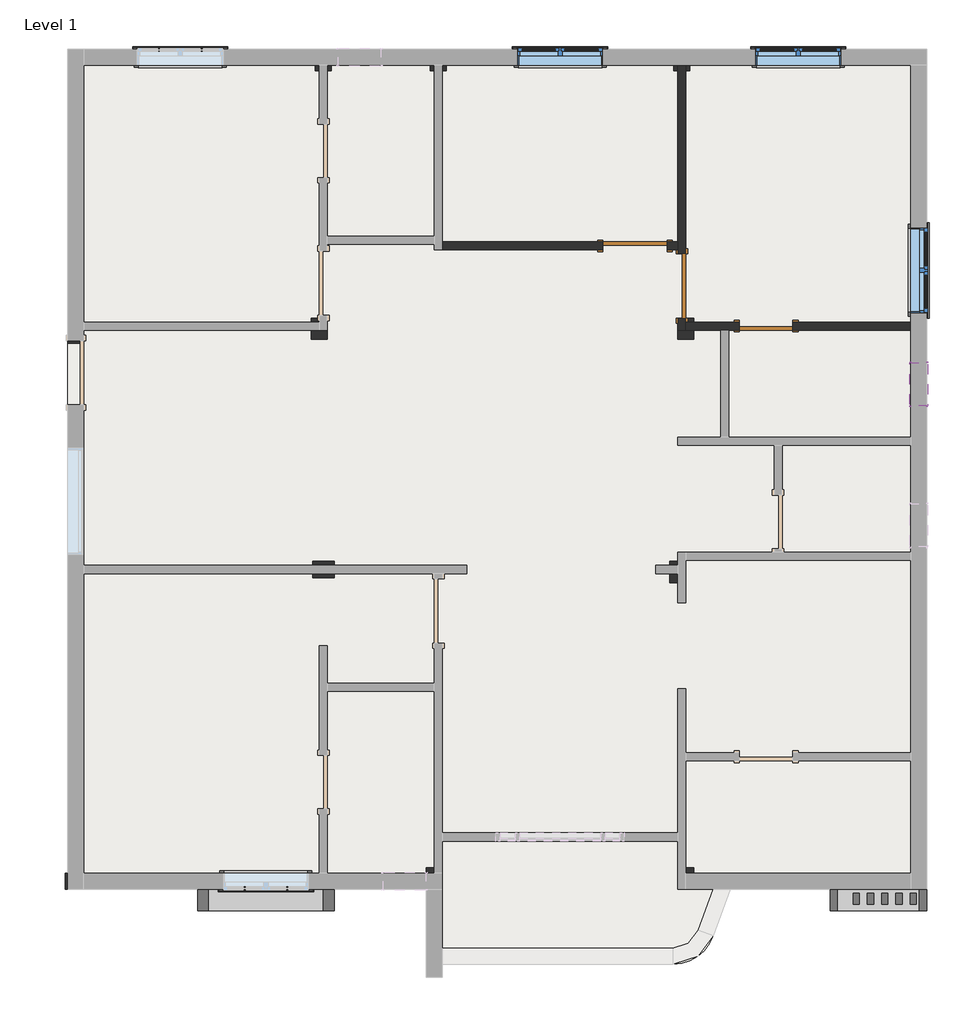
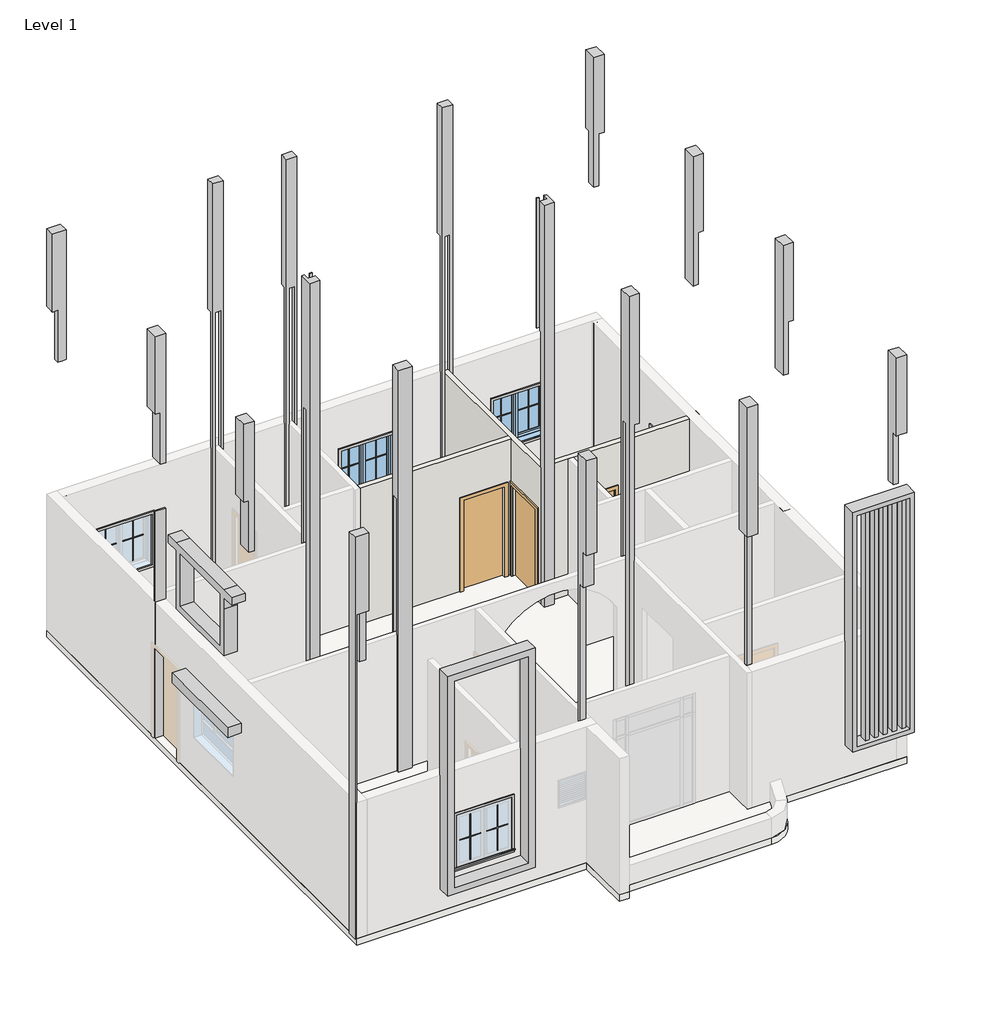
# One storey, part 2 of 2: 21 proxies, 17 columns, 4 windows, 3 doors, 3 walls, 1 slab.
"""IFC4 building model written with IfcOpenShell, lengths in millimetres."""

from ifc_helpers import new_model, si_unit, point, frame, frame_2d, origin, origin_with_axes, place, context, project, spatial, polyline, circle_curve, trimmed, segment, composite_curve, outline, extrude, faceted_brep, transform, mapped, element, save
from components import generic_models_1_generic_models_1_10505d45, muntin_pattern_2x2_muntin_pattern_2x2_4dfeb3f3, muntin_pattern_2x2_muntin_pattern_2x2_e852a7e4, trim_window_exterior_flat_with_sill_7cfdd449, trim_window_interior_flat_picture_frame_f1e0b15b, door_214872d5, door_e5f9f3c4, window_af3140d2, window_f2d8fef0

model = new_model("IFC4")

# Units and contexts
model_context = context("Model", 3, world=origin())
ifc_project = project(units=[si_unit("LENGTHUNIT", "METRE", prefix="MILLI")], contexts=[model_context])

# Site, building, storey
site = spatial("IfcSite", under=ifc_project)
building = spatial("IfcBuilding", under=site)
storey = spatial("IfcBuildingStorey", under=building, Name="Level 1", Elevation=0.0)

# Proxies
placement = place(None, origin())
generic_models_1_generic_models_1_shape = generic_models_1_generic_models_1_10505d45(model_context)
element("IfcBuildingElementProxy", 1, Name="Generic Models 1 : Generic Models 1", ObjectType="Generic Models 1 : Generic Models 1", at=placement, inside=storey, context=model_context, shape_type="MappedRepresentation", body=[
    mapped(generic_models_1_generic_models_1_shape, transform((0.0, 0.0, 0.0), x_axis=(1.0, 0.0, 0.0), y_axis=(0.0, 1.0, 0.0), z_axis=(0.0, 0.0, 1.0))),
])
muntin_pattern_2x2_muntin_pattern_2x2_shape = muntin_pattern_2x2_muntin_pattern_2x2_4dfeb3f3(model_context)
element("IfcBuildingElementProxy", 2, Name="Muntin Pattern_2x2 : Muntin Pattern_2x2", ObjectType="Muntin Pattern_2x2 : Muntin Pattern_2x2", at=placement, inside=storey, context=model_context, shape_type="MappedRepresentation", body=[
    mapped(muntin_pattern_2x2_muntin_pattern_2x2_shape, transform((-13598.9803125, 13522.091018, 984.25), x_axis=(1.0, 0.0, 0.0), y_axis=(0.0, 1.0, 0.0), z_axis=(0.0, 0.0, 1.0))),
])
element("IfcBuildingElementProxy", 3, Name="Muntin Pattern_2x2 : Muntin Pattern_2x2", ObjectType="Muntin Pattern_2x2 : Muntin Pattern_2x2", at=placement, inside=storey, context=model_context, shape_type="MappedRepresentation", body=[
    mapped(muntin_pattern_2x2_muntin_pattern_2x2_shape, transform((-8188.7803125, 13522.091018, 984.25), x_axis=(1.0, 0.0, 0.0), y_axis=(0.0, 1.0, 0.0), z_axis=(0.0, 0.0, 1.0))),
])
element("IfcBuildingElementProxy", 4, Name="Muntin Pattern_2x2 : Muntin Pattern_2x2", ObjectType="Muntin Pattern_2x2 : Muntin Pattern_2x2", at=placement, inside=storey, context=model_context, shape_type="MappedRepresentation", body=[
    mapped(muntin_pattern_2x2_muntin_pattern_2x2_shape, transform((-4797.8803125, 13522.091018, 984.25), x_axis=(1.0, 0.0, 0.0), y_axis=(0.0, 1.0, 0.0), z_axis=(0.0, 0.0, 1.0))),
])
element("IfcBuildingElementProxy", 5, Name="Muntin Pattern_2x2 : Muntin Pattern_2x2", ObjectType="Muntin Pattern_2x2 : Muntin Pattern_2x2", at=placement, inside=storey, context=model_context, shape_type="MappedRepresentation", body=[
    mapped(muntin_pattern_2x2_muntin_pattern_2x2_shape, transform((-2675.3928125, 10685.228518, 984.25), x_axis=(0.0, -1.0, 0.0), y_axis=(1.0, 0.0, 0.0), z_axis=(0.0, 0.0, 1.0))),
])
element("IfcBuildingElementProxy", 6, Name="Muntin Pattern_2x2 : Muntin Pattern_2x2", ObjectType="Muntin Pattern_2x2 : Muntin Pattern_2x2", at=placement, inside=storey, context=model_context, shape_type="MappedRepresentation", body=[
    mapped(muntin_pattern_2x2_muntin_pattern_2x2_shape, transform((-11773.3553125, 1577.741018, 984.25), x_axis=(-1.0, 0.0, 0.0), y_axis=(0.0, -1.0, 0.0), z_axis=(0.0, 0.0, 1.0))),
])
muntin_pattern_2x2_muntin_pattern_2x2_2_shape = muntin_pattern_2x2_muntin_pattern_2x2_e852a7e4(model_context)
element("IfcBuildingElementProxy", 7, Name="Muntin Pattern_2x2 : Muntin Pattern_2x2", ObjectType="Muntin Pattern_2x2 : Muntin Pattern_2x2", at=placement, inside=storey, context=model_context, shape_type="MappedRepresentation", body=[
    mapped(muntin_pattern_2x2_muntin_pattern_2x2_2_shape, transform((-12992.5553125, 13522.091018, 984.25), x_axis=(-1.0, 0.0, 0.0), y_axis=(0.0, -1.0, 0.0), z_axis=(0.0, 0.0, 1.0))),
])
element("IfcBuildingElementProxy", 8, Name="Muntin Pattern_2x2 : Muntin Pattern_2x2", ObjectType="Muntin Pattern_2x2 : Muntin Pattern_2x2", at=placement, inside=storey, context=model_context, shape_type="MappedRepresentation", body=[
    mapped(muntin_pattern_2x2_muntin_pattern_2x2_2_shape, transform((-7582.3553125, 13522.091018, 984.25), x_axis=(-1.0, 0.0, 0.0), y_axis=(0.0, -1.0, 0.0), z_axis=(0.0, 0.0, 1.0))),
])
element("IfcBuildingElementProxy", 9, Name="Muntin Pattern_2x2 : Muntin Pattern_2x2", ObjectType="Muntin Pattern_2x2 : Muntin Pattern_2x2", at=placement, inside=storey, context=model_context, shape_type="MappedRepresentation", body=[
    mapped(muntin_pattern_2x2_muntin_pattern_2x2_2_shape, transform((-4191.4553125, 13522.091018, 984.25), x_axis=(-1.0, 0.0, 0.0), y_axis=(0.0, -1.0, 0.0), z_axis=(0.0, 0.0, 1.0))),
])
element("IfcBuildingElementProxy", 10, Name="Muntin Pattern_2x2 : Muntin Pattern_2x2", ObjectType="Muntin Pattern_2x2 : Muntin Pattern_2x2", at=placement, inside=storey, context=model_context, shape_type="MappedRepresentation", body=[
    mapped(muntin_pattern_2x2_muntin_pattern_2x2_2_shape, transform((-2675.3928125, 10078.803518, 984.25), x_axis=(0.0, 1.0, 0.0), y_axis=(-1.0, 0.0, 0.0), z_axis=(0.0, 0.0, 1.0))),
])
element("IfcBuildingElementProxy", 11, Name="Muntin Pattern_2x2 : Muntin Pattern_2x2", ObjectType="Muntin Pattern_2x2 : Muntin Pattern_2x2", at=placement, inside=storey, context=model_context, shape_type="MappedRepresentation", body=[
    mapped(muntin_pattern_2x2_muntin_pattern_2x2_2_shape, transform((-12379.7803125, 1577.741018, 984.25), x_axis=(1.0, 0.0, 0.0), y_axis=(0.0, 1.0, 0.0), z_axis=(0.0, 0.0, 1.0))),
])
trim_window_exterior_flat_with_sill_shape = trim_window_exterior_flat_with_sill_7cfdd449(model_context)
element("IfcBuildingElementProxy", 12, Name="Trim-Window-Exterior-Flat : with Sill", ObjectType="Trim-Window-Exterior-Flat : with Sill", at=placement, inside=storey, context=model_context, shape_type="MappedRepresentation", body=[
    mapped(trim_window_exterior_flat_with_sill_shape, transform((-13295.7678125, 13531.616018, 2133.6), x_axis=(-1.0, 0.0, 0.0), y_axis=(0.0, 0.0, 1.0), z_axis=(0.0, 1.0, 0.0))),
])
element("IfcBuildingElementProxy", 13, Name="Trim-Window-Exterior-Flat : with Sill", ObjectType="Trim-Window-Exterior-Flat : with Sill", at=placement, inside=storey, context=model_context, shape_type="MappedRepresentation", body=[
    mapped(trim_window_exterior_flat_with_sill_shape, transform((-7885.5678125, 13531.616018, 2133.6), x_axis=(-1.0, 0.0, 0.0), y_axis=(0.0, 0.0, 1.0), z_axis=(0.0, 1.0, 0.0))),
])
element("IfcBuildingElementProxy", 14, Name="Trim-Window-Exterior-Flat : with Sill", ObjectType="Trim-Window-Exterior-Flat : with Sill", at=placement, inside=storey, context=model_context, shape_type="MappedRepresentation", body=[
    mapped(trim_window_exterior_flat_with_sill_shape, transform((-4494.6678125, 13531.616018, 2133.6), x_axis=(-1.0, 0.0, 0.0), y_axis=(0.0, 0.0, 1.0), z_axis=(0.0, 1.0, 0.0))),
])
element("IfcBuildingElementProxy", 15, Name="Trim-Window-Exterior-Flat : with Sill", ObjectType="Trim-Window-Exterior-Flat : with Sill", at=placement, inside=storey, context=model_context, shape_type="MappedRepresentation", body=[
    mapped(trim_window_exterior_flat_with_sill_shape, transform((-2665.8678125, 10382.016018, 2133.6), x_axis=(0.0, 1.0, 0.0), y_axis=(0.0, 0.0, 1.0), z_axis=(1.0, 0.0, 0.0))),
])
element("IfcBuildingElementProxy", 16, Name="Trim-Window-Exterior-Flat : with Sill", ObjectType="Trim-Window-Exterior-Flat : with Sill", at=placement, inside=storey, context=model_context, shape_type="MappedRepresentation", body=[
    mapped(trim_window_exterior_flat_with_sill_shape, transform((-12076.5678125, 1568.216018, 2133.6), x_axis=(1.0, 0.0, 0.0), y_axis=(0.0, 0.0, 1.0), z_axis=(0.0, -1.0, 0.0))),
])
trim_window_interior_flat_picture_frame_shape = trim_window_interior_flat_picture_frame_f1e0b15b(model_context)
element("IfcBuildingElementProxy", 17, Name="Trim-Window-Interior-Flat : Picture Frame", ObjectType="Trim-Window-Interior-Flat : Picture Frame", at=placement, inside=storey, context=model_context, shape_type="MappedRepresentation", body=[
    mapped(trim_window_interior_flat_picture_frame_shape, transform((-13295.7678125, 13303.016018, 2133.6), x_axis=(1.0, 0.0, 0.0), y_axis=(0.0, 0.0, 1.0), z_axis=(0.0, -1.0, 0.0))),
])
element("IfcBuildingElementProxy", 18, Name="Trim-Window-Interior-Flat : Picture Frame", ObjectType="Trim-Window-Interior-Flat : Picture Frame", at=placement, inside=storey, context=model_context, shape_type="MappedRepresentation", body=[
    mapped(trim_window_interior_flat_picture_frame_shape, transform((-7885.5678125, 13303.016018, 2133.6), x_axis=(1.0, 0.0, 0.0), y_axis=(0.0, 0.0, 1.0), z_axis=(0.0, -1.0, 0.0))),
])
element("IfcBuildingElementProxy", 19, Name="Trim-Window-Interior-Flat : Picture Frame", ObjectType="Trim-Window-Interior-Flat : Picture Frame", at=placement, inside=storey, context=model_context, shape_type="MappedRepresentation", body=[
    mapped(trim_window_interior_flat_picture_frame_shape, transform((-4494.6678125, 13303.016018, 2133.6), x_axis=(1.0, 0.0, 0.0), y_axis=(0.0, 0.0, 1.0), z_axis=(0.0, -1.0, 0.0))),
])
element("IfcBuildingElementProxy", 20, Name="Trim-Window-Interior-Flat : Picture Frame", ObjectType="Trim-Window-Interior-Flat : Picture Frame", at=placement, inside=storey, context=model_context, shape_type="MappedRepresentation", body=[
    mapped(trim_window_interior_flat_picture_frame_shape, transform((-2894.4678125, 10382.016018, 2133.6), x_axis=(0.0, -1.0, 0.0), y_axis=(0.0, 0.0, 1.0), z_axis=(-1.0, 0.0, 0.0))),
])
element("IfcBuildingElementProxy", 21, Name="Trim-Window-Interior-Flat : Picture Frame", ObjectType="Trim-Window-Interior-Flat : Picture Frame", at=placement, inside=storey, context=model_context, shape_type="MappedRepresentation", body=[
    mapped(trim_window_interior_flat_picture_frame_shape, transform((-12076.5678125, 1796.816018, 2133.6), x_axis=(-1.0, 0.0, 0.0), y_axis=(0.0, 0.0, 1.0), z_axis=(0.0, 1.0, 0.0))),
])

# Columns
element("IfcColumn", 22, ObjectType="Rectangular Column : 9\" x 12\"", at=placement, inside=storey, context=model_context, shape_type="Brep", body=[
    faceted_brep([(-14591.1678125, 13531.616018, 0.0), (-14591.1678125, 13303.016018, 0.0), (-14667.3678125, 13303.016018, 0.0), (-14667.3678125, 13531.616018, 0.0), (-14667.3678125, 13303.016018, 3200.4), (-14667.3678125, 13531.616018, 3200.4), (-14591.1678125, 13303.016018, 3200.4), (-14591.1678125, 13531.616018, 3200.4)], [[[0, 1, 2, 3]], [[3, 2, 4, 5]], [[6, 7, 5, 4]], [[1, 0, 7, 6]], [[2, 1, 6, 4]], [[0, 3, 5, 7]]]),
    faceted_brep([(-14591.1678125, 13531.616018, 9448.8), (-14591.1678125, 13303.016018, 9448.8), (-14591.1678125, 13303.016018, 6400.8), (-14591.1678125, 13417.316018, 6400.8), (-14591.1678125, 13417.316018, 7620.0), (-14591.1678125, 13531.616018, 7620.0), (-14895.9678125, 13303.016018, 9448.8), (-14895.9678125, 13303.016018, 7620.0), (-14781.6678125, 13303.016018, 7620.0), (-14781.6678125, 13303.016018, 6400.8), (-14667.3678125, 13303.016018, 6400.8), (-14895.9678125, 13531.616018, 9448.8), (-14895.9678125, 13531.616018, 7620.0), (-14895.9678125, 13417.316018, 7620.0), (-14781.6678125, 13417.316018, 6400.8), (-14667.3678125, 13417.316018, 6400.8), (-14781.6678125, 13417.316018, 7620.0)], [[[0, 1, 2, 3, 4, 5]], [[1, 6, 7, 8, 9, 10, 2]], [[6, 11, 12, 13, 7]], [[11, 0, 5, 12]], [[1, 0, 11, 6]], [[10, 9, 14, 15]], [[2, 10, 15, 3]], [[8, 16, 14, 9]], [[16, 8, 7, 13]], [[16, 4, 3, 15, 14]], [[4, 16, 13, 12, 5]]]),
])
element("IfcColumn", 23, ObjectType="Rectangular Column : 9\" x 12\"", at=placement, inside=storey, context=model_context, shape_type="Brep", body=[
    faceted_brep([(-11371.7178125, 13226.816018, 0.0), (-11371.7178125, 13303.016018, 0.0), (-11314.5678125, 13303.016018, 0.0), (-11314.5678125, 13226.816018, 0.0), (-11143.1178125, 13226.816018, 9448.8), (-11143.1178125, 13226.816018, 0.0), (-11143.1178125, 13303.016018, 0.0), (-11143.1178125, 13303.016018, 3200.4), (-11143.1178125, 13303.016018, 6400.8), (-11143.1178125, 13417.316018, 6400.8), (-11143.1178125, 13417.316018, 9448.8), (-11257.4178125, 13226.816018, 9448.8), (-11371.7178125, 13226.816018, 9448.8), (-11371.7178125, 13226.816018, 6400.8), (-11314.5678125, 13226.816018, 3200.4), (-11314.5678125, 13226.816018, 6400.8), (-11257.4178125, 13226.816018, 6400.8), (-11200.2678125, 13226.816018, 6400.8), (-11200.2678125, 13226.816018, 3200.4), (-11200.2678125, 13226.816018, 0.0), (-11371.7178125, 13417.316018, 9448.8), (-11371.7178125, 13417.316018, 6400.8), (-11371.7178125, 13303.016018, 6400.8), (-11371.7178125, 13303.016018, 3200.4), (-11314.5678125, 13303.016018, 3200.4), (-11200.2678125, 13303.016018, 0.0), (-11200.2678125, 13303.016018, 3200.4), (-11314.5678125, 13303.016018, 6400.8), (-11200.2678125, 13303.016018, 6400.8)], [[[0, 1, 2, 3]], [[4, 5, 6, 7, 8, 9, 10]], [[5, 4, 11, 12, 13, 0, 3, 14, 15, 16, 17, 18, 19]], [[0, 13, 12, 20, 21, 22, 23, 1]], [[12, 11, 4, 10, 20]], [[1, 23, 24, 2]], [[3, 2, 24, 14]], [[25, 19, 18, 26]], [[6, 5, 19, 25]], [[7, 6, 25, 26]], [[23, 22, 27, 24]], [[27, 22, 21, 9, 8, 28]], [[27, 15, 14, 24]], [[17, 28, 26, 18]], [[15, 27, 28, 17, 16]], [[8, 7, 26, 28]], [[10, 9, 21, 20]]]),
])
element("IfcColumn", 24, ObjectType="Rectangular Column : 9\" x 12\"", at=placement, inside=storey, context=model_context, shape_type="Brep", body=[
    faceted_brep([(-9733.4178125, 13226.816018, 0.0), (-9733.4178125, 13303.016018, 0.0), (-9676.2678125, 13303.016018, 0.0), (-9676.2678125, 13226.816018, 0.0), (-9504.8178125, 13226.816018, 9448.8), (-9504.8178125, 13226.816018, 0.0), (-9504.8178125, 13303.016018, 0.0), (-9504.8178125, 13303.016018, 3200.4), (-9504.8178125, 13303.016018, 6400.8), (-9504.8178125, 13417.316018, 6400.8), (-9504.8178125, 13417.316018, 9448.8), (-9733.4178125, 13226.816018, 9448.8), (-9676.2678125, 13226.816018, 3200.4), (-9676.2678125, 13226.816018, 6400.8), (-9561.9678125, 13226.816018, 6400.8), (-9561.9678125, 13226.816018, 3200.4), (-9561.9678125, 13226.816018, 0.0), (-9733.4178125, 13417.316018, 9448.8), (-9733.4178125, 13417.316018, 6400.8), (-9733.4178125, 13303.016018, 6400.8), (-9733.4178125, 13303.016018, 3200.4), (-9676.2678125, 13303.016018, 3200.4), (-9561.9678125, 13303.016018, 0.0), (-9561.9678125, 13303.016018, 3200.4), (-9676.2678125, 13303.016018, 6400.8), (-9561.9678125, 13303.016018, 6400.8)], [[[0, 1, 2, 3]], [[4, 5, 6, 7, 8, 9, 10]], [[5, 4, 11, 0, 3, 12, 13, 14, 15, 16]], [[0, 11, 17, 18, 19, 20, 1]], [[11, 4, 10, 17]], [[1, 20, 21, 2]], [[3, 2, 21, 12]], [[22, 16, 15, 23]], [[6, 5, 16, 22]], [[7, 6, 22, 23]], [[20, 19, 24, 21]], [[24, 19, 18, 9, 8, 25]], [[24, 13, 12, 21]], [[14, 25, 23, 15]], [[13, 24, 25, 14]], [[8, 7, 23, 25]], [[10, 9, 18, 17]]]),
])
element("IfcColumn", 25, ObjectType="Rectangular Column : 9\" x 12\"", at=placement, inside=storey, context=model_context, shape_type="Brep", body=[
    faceted_brep([(-6266.3178125, 13226.816018, 0.0), (-6266.3178125, 13303.016018, 0.0), (-6209.1678125, 13303.016018, 0.0), (-6209.1678125, 13226.816018, 0.0), (-6037.7178125, 13226.816018, 9448.8), (-6037.7178125, 13226.816018, 6400.8), (-6037.7178125, 13226.816018, 0.0), (-6037.7178125, 13303.016018, 0.0), (-6037.7178125, 13303.016018, 3200.4), (-6037.7178125, 13303.016018, 6400.8), (-6037.7178125, 13417.316018, 6400.8), (-6037.7178125, 13417.316018, 9448.8), (-6152.0178125, 13226.816018, 9448.8), (-6266.3178125, 13226.816018, 9448.8), (-6209.1678125, 13226.816018, 3200.4), (-6209.1678125, 13226.816018, 6400.8), (-6152.0178125, 13226.816018, 6400.8), (-6094.8678125, 13226.816018, 6400.8), (-6094.8678125, 13226.816018, 3200.4), (-6094.8678125, 13226.816018, 0.0), (-6266.3178125, 13417.316018, 9448.8), (-6266.3178125, 13417.316018, 6400.8), (-6266.3178125, 13303.016018, 6400.8), (-6266.3178125, 13303.016018, 3200.4), (-6209.1678125, 13303.016018, 3200.4), (-6094.8678125, 13303.016018, 0.0), (-6094.8678125, 13303.016018, 3200.4), (-6209.1678125, 13303.016018, 6400.8), (-6094.8678125, 13303.016018, 6400.8)], [[[0, 1, 2, 3]], [[4, 5, 6, 7, 8, 9, 10, 11]], [[6, 5, 4, 12, 13, 0, 3, 14, 15, 16, 17, 18, 19]], [[0, 13, 20, 21, 22, 23, 1]], [[13, 12, 4, 11, 20]], [[1, 23, 24, 2]], [[3, 2, 24, 14]], [[25, 19, 18, 26]], [[7, 6, 19, 25]], [[8, 7, 25, 26]], [[23, 22, 27, 24]], [[27, 22, 21, 10, 9, 28]], [[27, 15, 14, 24]], [[17, 28, 26, 18]], [[15, 27, 28, 17, 16]], [[9, 8, 26, 28]], [[11, 10, 21, 20]]]),
])
element("IfcColumn", 26, ObjectType="Rectangular Column : 9\" x 12\"", at=placement, inside=storey, context=model_context, shape_type="Brep", body=[
    faceted_brep([(-2665.8678125, 13226.816018, 0.0), (-2894.4678125, 13226.816018, 0.0), (-2894.4678125, 13303.016018, 0.0), (-2665.8678125, 13303.016018, 0.0), (-2894.4678125, 13303.016018, 3200.4), (-2665.8678125, 13303.016018, 3200.4), (-2665.8678125, 13226.816018, 3200.4), (-2894.4678125, 13226.816018, 3200.4)], [[[0, 1, 2, 3]], [[3, 2, 4, 5]], [[6, 5, 4, 7]], [[0, 3, 5, 6]], [[1, 0, 6, 7]], [[2, 1, 7, 4]]]),
    faceted_brep([(-2894.4678125, 13531.616018, 9448.8), (-2665.8678125, 13531.616018, 9448.8), (-2665.8678125, 13531.616018, 7620.0), (-2894.4678125, 13531.616018, 7620.0), (-2665.8678125, 13226.816018, 9448.8), (-2665.8678125, 13226.816018, 7620.0), (-2665.8678125, 13417.316018, 7620.0), (-2894.4678125, 13226.816018, 9448.8), (-2894.4678125, 13226.816018, 6400.8), (-2780.1678125, 13226.816018, 6400.8), (-2780.1678125, 13226.816018, 7620.0), (-2894.4678125, 13417.316018, 7620.0), (-2894.4678125, 13417.316018, 6400.8), (-2894.4678125, 13303.016018, 6400.8), (-2780.1678125, 13417.316018, 6400.8), (-2780.1678125, 13303.016018, 6400.8), (-2780.1678125, 13417.316018, 7620.0)], [[[0, 1, 2, 3]], [[1, 4, 5, 6, 2]], [[4, 7, 8, 9, 10, 5]], [[7, 0, 3, 11, 12, 13, 8]], [[1, 0, 7, 4]], [[13, 12, 14, 15]], [[8, 13, 15, 9]], [[12, 11, 16, 14]], [[3, 2, 6, 16, 11]], [[16, 10, 9, 15, 14]], [[10, 16, 6, 5]]]),
])
element("IfcColumn", 27, ObjectType="Rectangular Column : 9\" x 12\"", at=placement, inside=storey, context=model_context, shape_type="Brep", body=[
    faceted_brep([(-14895.9678125, 9645.416018, 0.0), (-14667.3678125, 9645.416018, 0.0), (-14667.3678125, 9531.116018, 0.0), (-14667.3678125, 9340.616018, 0.0), (-14895.9678125, 9340.616018, 0.0), (-14895.9678125, 9378.716018, 3200.4), (-14667.3678125, 9378.716018, 3200.4), (-14667.3678125, 9531.116018, 3200.4), (-14667.3678125, 9645.416018, 3200.4), (-14895.9678125, 9645.416018, 3200.4), (-14895.9678125, 9378.716018, 5334.0), (-14667.3678125, 9378.716018, 5334.0), (-14895.9678125, 9340.616018, 5334.0), (-14667.3678125, 9340.616018, 5334.0)], [[[0, 1, 2, 3, 4]], [[5, 6, 7, 8, 9]], [[6, 5, 10, 11]], [[11, 10, 12, 13]], [[1, 0, 9, 8]], [[3, 2, 1, 8, 7, 6, 11, 13]], [[4, 3, 13, 12]], [[0, 4, 12, 10, 5, 9]]]),
    faceted_brep([(-14895.9678125, 9645.416018, 9448.8), (-14667.3678125, 9645.416018, 9448.8), (-14667.3678125, 9645.416018, 6400.8), (-14781.6678125, 9645.416018, 6400.8), (-14781.6678125, 9645.416018, 7620.0), (-14895.9678125, 9645.416018, 7620.0), (-14667.3678125, 9340.616018, 9448.8), (-14667.3678125, 9340.616018, 6400.8), (-14895.9678125, 9340.616018, 9448.8), (-14895.9678125, 9340.616018, 7620.0), (-14781.6678125, 9340.616018, 7620.0), (-14781.6678125, 9340.616018, 6400.8)], [[[0, 1, 2, 3, 4, 5]], [[1, 6, 7, 2]], [[6, 8, 9, 10, 11, 7]], [[8, 0, 5, 9]], [[1, 0, 8, 6]], [[2, 7, 11, 3]], [[10, 4, 3, 11]], [[4, 10, 9, 5]]]),
])
element("IfcColumn", 28, ObjectType="Rectangular Column : 9\" x 12\"", at=placement, inside=storey, context=model_context, shape_type="Brep", body=[
    faceted_brep([(-11200.2678125, 9397.766018, 0.0), (-11428.8678125, 9397.766018, 0.0), (-11428.8678125, 9531.116018, 0.0), (-11314.5678125, 9531.116018, 0.0), (-11200.2678125, 9531.116018, 0.0), (-11200.2678125, 9397.766018, 9448.8), (-11200.2678125, 9531.116018, 3200.4), (-11200.2678125, 9531.116018, 6400.8), (-11200.2678125, 9569.216018, 6400.8), (-11200.2678125, 9569.216018, 9448.8), (-11428.8678125, 9397.766018, 9448.8), (-11428.8678125, 9702.566018, 9448.8), (-11428.8678125, 9702.566018, 0.0), (-11428.8678125, 9645.416018, 0.0), (-11428.8678125, 9645.416018, 3200.4), (-11428.8678125, 9645.416018, 6400.8), (-11428.8678125, 9531.116018, 6400.8), (-11428.8678125, 9531.116018, 3200.4), (-11314.5678125, 9702.566018, 0.0), (-11314.5678125, 9702.566018, 3200.4), (-11314.5678125, 9645.416018, 3200.4), (-11314.5678125, 9645.416018, 0.0), (-11314.5678125, 9531.116018, 3200.4), (-11314.5678125, 9702.566018, 6400.8), (-11314.5678125, 9645.416018, 6400.8), (-11314.5678125, 9531.116018, 6400.8), (-11314.5678125, 9569.216018, 6400.8), (-11257.4178125, 9569.216018, 6400.8), (-11371.7178125, 9645.416018, 6400.8), (-11371.7178125, 9569.216018, 6400.8), (-11371.7178125, 9702.566018, 6400.8), (-11371.7178125, 9702.566018, 9448.8), (-11371.7178125, 9569.216018, 9448.8), (-11257.4178125, 9569.216018, 9448.8)], [[[0, 1, 2, 3, 4]], [[5, 0, 4, 6, 7, 8, 9]], [[1, 0, 5, 10]], [[11, 12, 13, 14, 15, 16, 17, 2, 1, 10]], [[18, 19, 20, 21]], [[4, 3, 22, 6]], [[3, 2, 17, 22]], [[13, 21, 20, 14]], [[12, 18, 21, 13]], [[19, 23, 24, 20]], [[7, 25, 26, 27, 8]], [[25, 7, 6, 22]], [[16, 25, 22, 17]], [[15, 14, 20, 24, 28]], [[25, 16, 15, 28, 29, 26]], [[28, 30, 31, 32, 29]], [[30, 28, 24, 23]], [[29, 32, 33, 27, 26]], [[9, 8, 27, 33]], [[12, 11, 31, 30, 23, 19, 18]], [[10, 5, 9, 33, 32, 31, 11]]]),
    faceted_brep([(-11200.2678125, 9702.566018, 9448.8), (-11200.2678125, 9702.566018, 6400.8), (-11257.4178125, 9702.566018, 6400.8), (-11257.4178125, 9702.566018, 9448.8), (-11257.4178125, 9683.516018, 9448.8), (-11200.2678125, 9683.516018, 9448.8), (-11257.4178125, 9683.516018, 6400.8), (-11200.2678125, 9683.516018, 6400.8)], [[[0, 1, 2, 3]], [[0, 3, 4, 5]], [[3, 2, 6, 4]], [[7, 5, 4, 6]], [[2, 1, 7, 6]], [[1, 0, 5, 7]]]),
])
element("IfcColumn", 29, ObjectType="Rectangular Column : 9\" x 12\"", at=placement, inside=storey, context=model_context, shape_type="Brep", body=[
    faceted_brep([(-5980.5678125, 9397.766018, 0.0), (-6209.1678125, 9397.766018, 0.0), (-6209.1678125, 9531.116018, 0.0), (-6094.8678125, 9531.116018, 0.0), (-5980.5678125, 9531.116018, 0.0), (-5980.5678125, 9702.566018, 9448.8), (-5980.5678125, 9702.566018, 0.0), (-6094.8678125, 9702.566018, 0.0), (-6094.8678125, 9702.566018, 2133.6), (-6094.8678125, 9702.566018, 3200.4), (-6094.8678125, 9702.566018, 5334.0), (-6094.8678125, 9702.566018, 6400.8), (-6037.7178125, 9702.566018, 6400.8), (-6037.7178125, 9702.566018, 9448.8), (-5980.5678125, 9397.766018, 9448.8), (-5980.5678125, 9531.116018, 3200.4), (-5980.5678125, 9531.116018, 6400.8), (-5980.5678125, 9645.416018, 6400.8), (-5980.5678125, 9645.416018, 3200.4), (-5980.5678125, 9645.416018, 0.0), (-6209.1678125, 9397.766018, 9448.8), (-6209.1678125, 9569.216018, 9448.8), (-6209.1678125, 9569.216018, 6400.8), (-6209.1678125, 9531.116018, 6400.8), (-6209.1678125, 9531.116018, 3200.4), (-6094.8678125, 9645.416018, 0.0), (-6094.8678125, 9645.416018, 3200.4), (-6094.8678125, 9531.116018, 3200.4), (-6094.8678125, 9645.416018, 6400.8), (-6094.8678125, 9683.516018, 6400.8), (-6094.8678125, 9531.116018, 6400.8), (-6094.8678125, 9569.216018, 6400.8), (-6037.7178125, 9645.416018, 6400.8), (-6037.7178125, 9569.216018, 6400.8), (-6037.7178125, 9569.216018, 9448.8), (-6037.7178125, 9683.516018, 6400.8), (-6037.7178125, 9683.516018, 9448.8)], [[[0, 1, 2, 3, 4]], [[5, 6, 7, 8, 9, 10, 11, 12, 13]], [[6, 5, 14, 0, 4, 15, 16, 17, 18, 19]], [[1, 0, 14, 20]], [[1, 20, 21, 22, 23, 24, 2]], [[8, 7, 25, 26, 9]], [[3, 2, 24, 27]], [[4, 3, 27, 15]], [[25, 19, 18, 26]], [[7, 6, 19, 25]], [[10, 9, 26, 28, 29, 11]], [[30, 23, 22, 31]], [[23, 30, 27, 24]], [[30, 16, 15, 27]], [[18, 17, 32, 28, 26]], [[16, 30, 31, 33, 32, 17]], [[22, 21, 34, 33, 31]], [[29, 28, 32, 35]], [[33, 34, 36, 35, 32]], [[12, 35, 36, 13]], [[35, 12, 11, 29]], [[14, 5, 13, 36, 34, 21, 20]]]),
    faceted_brep([(-6209.1678125, 9702.566018, 9448.8), (-6209.1678125, 9683.516018, 9448.8), (-6152.0178125, 9683.516018, 9448.8), (-6152.0178125, 9702.566018, 9448.8), (-6209.1678125, 9683.516018, 6400.8), (-6152.0178125, 9683.516018, 6400.8), (-6209.1678125, 9702.566018, 6400.8), (-6152.0178125, 9702.566018, 6400.8)], [[[0, 1, 2, 3]], [[1, 4, 5, 2]], [[4, 6, 7, 5]], [[7, 3, 2, 5]], [[0, 6, 4, 1]], [[6, 0, 3, 7]]]),
])
element("IfcColumn", 30, ObjectType="Rectangular Column : 9\" x 12\"", at=placement, inside=storey, context=model_context, shape_type="Brep", body=[
    faceted_brep([(-2894.4678125, 9702.566018, 0.0), (-2665.8678125, 9702.566018, 0.0), (-2665.8678125, 9397.766018, 0.0), (-2894.4678125, 9397.766018, 0.0), (-2894.4678125, 9531.116018, 0.0), (-2894.4678125, 9645.416018, 0.0), (-2665.8678125, 9702.566018, 3200.4), (-2894.4678125, 9702.566018, 3200.4), (-2894.4678125, 9645.416018, 3200.4), (-2894.4678125, 9531.116018, 3200.4), (-2894.4678125, 9397.766018, 3200.4), (-2665.8678125, 9397.766018, 3200.4)], [[[0, 1, 2, 3, 4, 5]], [[6, 7, 8, 9, 10, 11]], [[1, 0, 7, 6]], [[2, 1, 6, 11]], [[3, 2, 11, 10]], [[0, 5, 4, 3, 10, 9, 8, 7]]]),
    faceted_brep([(-2894.4678125, 9702.566018, 9448.8), (-2665.8678125, 9702.566018, 9448.8), (-2665.8678125, 9702.566018, 7620.0), (-2780.1678125, 9702.566018, 7620.0), (-2780.1678125, 9702.566018, 6400.8), (-2894.4678125, 9702.566018, 6400.8), (-2665.8678125, 9397.766018, 9448.8), (-2665.8678125, 9397.766018, 7620.0), (-2894.4678125, 9397.766018, 9448.8), (-2894.4678125, 9397.766018, 6400.8), (-2780.1678125, 9397.766018, 6400.8), (-2780.1678125, 9397.766018, 7620.0)], [[[0, 1, 2, 3, 4, 5]], [[1, 6, 7, 2]], [[6, 8, 9, 10, 11, 7]], [[8, 0, 5, 9]], [[1, 0, 8, 6]], [[9, 5, 4, 10]], [[3, 11, 10, 4]], [[11, 3, 2, 7]]]),
])
element("IfcColumn", 31, ObjectType="Rectangular Column : 9\" x 12\"", at=placement, inside=storey, context=model_context, shape_type="Brep", body=[
    faceted_brep([(-14895.9678125, 6235.466018, 0.0), (-14667.3678125, 6235.466018, 0.0), (-14667.3678125, 6178.316018, 0.0), (-14667.3678125, 6064.016018, 0.0), (-14667.3678125, 5930.666018, 0.0), (-14895.9678125, 5930.666018, 0.0), (-14667.3678125, 6235.466018, 3200.4), (-14895.9678125, 6235.466018, 3200.4), (-14895.9678125, 5930.666018, 3200.4), (-14667.3678125, 5930.666018, 3200.4), (-14667.3678125, 6064.016018, 3200.4), (-14667.3678125, 6178.316018, 3200.4)], [[[0, 1, 2, 3, 4, 5]], [[6, 7, 8, 9, 10, 11]], [[1, 0, 7, 6]], [[4, 3, 2, 1, 6, 11, 10, 9]], [[5, 4, 9, 8]], [[0, 5, 8, 7]]]),
    faceted_brep([(-14895.9678125, 6235.466018, 9448.8), (-14667.3678125, 6235.466018, 9448.8), (-14667.3678125, 6235.466018, 6400.8), (-14781.6678125, 6235.466018, 6400.8), (-14781.6678125, 6235.466018, 7620.0), (-14895.9678125, 6235.466018, 7620.0), (-14667.3678125, 5930.666018, 9448.8), (-14667.3678125, 5930.666018, 6400.8), (-14895.9678125, 5930.666018, 9448.8), (-14895.9678125, 5930.666018, 7620.0), (-14781.6678125, 5930.666018, 7620.0), (-14781.6678125, 5930.666018, 6400.8)], [[[0, 1, 2, 3, 4, 5]], [[1, 6, 7, 2]], [[6, 8, 9, 10, 11, 7]], [[8, 0, 5, 9]], [[1, 0, 8, 6]], [[2, 7, 11, 3]], [[10, 4, 3, 11]], [[4, 10, 9, 5]]]),
])
element("IfcColumn", 32, ObjectType="Rectangular Column : 9\" x 12\"", at=placement, inside=storey, context=model_context, shape_type="SweptSolid", body=[
    extrude(outline(polyline([(6006.866018, 0.0), (6006.866018, 9448.8), (6235.466018, 9448.8), (6235.466018, 0.0), (6178.316018, 0.0), (6178.316018, 3200.4), (6178.316018, 6400.8), (6064.016018, 6400.8), (6064.016018, 3200.4), (6064.016018, 0.0), (6006.866018, 0.0)])), frame((-11409.8178125, 0.0, 0.0), z_axis=(1.0, 0.0, 0.0), x_axis=(0.0, 1.0, 0.0)), (0.0, 0.0, 1.0), 304.8),
])
element("IfcColumn", 33, ObjectType="Rectangular Column : 9\" x 12\"", at=placement, inside=storey, context=model_context, shape_type="Brep", body=[
    faceted_brep([(-6323.4678125, 5930.666018, 0.0), (-6323.4678125, 6064.016018, 0.0), (-6209.1678125, 6064.016018, 0.0), (-6209.1678125, 5930.666018, 0.0), (-6323.4678125, 6235.466018, 9448.8), (-6094.8678125, 6235.466018, 9448.8), (-6094.8678125, 6235.466018, 6400.8), (-6209.1678125, 6235.466018, 6400.8), (-6209.1678125, 6235.466018, 3200.4), (-6209.1678125, 6235.466018, 0.0), (-6323.4678125, 6235.466018, 0.0), (-6094.8678125, 5930.666018, 9448.8), (-6094.8678125, 5930.666018, 6400.8), (-6323.4678125, 5930.666018, 9448.8), (-6209.1678125, 5930.666018, 3200.4), (-6209.1678125, 5930.666018, 6400.8), (-6323.4678125, 6178.316018, 0.0), (-6323.4678125, 6178.316018, 3200.4), (-6323.4678125, 6178.316018, 6400.8), (-6323.4678125, 6064.016018, 6400.8), (-6323.4678125, 6064.016018, 3200.4), (-6209.1678125, 6064.016018, 3200.4), (-6209.1678125, 6178.316018, 0.0), (-6209.1678125, 6178.316018, 3200.4), (-6209.1678125, 6064.016018, 6400.8), (-6209.1678125, 6178.316018, 6400.8)], [[[0, 1, 2, 3]], [[4, 5, 6, 7, 8, 9, 10]], [[5, 11, 12, 6]], [[11, 13, 0, 3, 14, 15, 12]], [[4, 10, 16, 17, 18, 19, 20, 1, 0, 13]], [[5, 4, 13, 11]], [[2, 1, 20, 21]], [[16, 22, 23, 17]], [[22, 9, 8, 23]], [[22, 16, 10, 9]], [[3, 2, 21, 14]], [[19, 24, 21, 20]], [[25, 18, 17, 23]], [[24, 19, 18, 25]], [[7, 25, 23, 8]], [[25, 7, 6, 12, 15, 24]], [[24, 15, 14, 21]]]),
])
element("IfcColumn", 34, ObjectType="Rectangular Column : 9\" x 12\"", at=placement, inside=storey, context=model_context, shape_type="SweptSolid", body=[
    extrude(outline(polyline([(-2894.4678125, 6235.466018), (-2665.8678125, 6235.466018), (-2665.8678125, 5930.666018), (-2894.4678125, 5930.666018), (-2894.4678125, 6235.466018)])), origin_with_axes(), (0.0, 0.0, 1.0), 3200.4),
    extrude(outline(polyline([(9448.8, -2665.8678125), (9448.8, -2894.4678125), (6400.8, -2894.4678125), (6400.8, -2780.1678125), (7620.0, -2780.1678125), (7620.0, -2665.8678125), (9448.8, -2665.8678125)])), frame((0.0, 5930.666018, 0.0), z_axis=(0.0, 1.0, 0.0), x_axis=(0.0, 0.0, 1.0)), (0.0, 0.0, 1.0), 304.8),
])
element("IfcColumn", 35, ObjectType="Rectangular Column : 9\" x 12\"", at=placement, inside=storey, context=model_context, shape_type="Brep", body=[
    faceted_brep([(-14934.0678125, 1568.216018, 0.0), (-14934.0678125, 1796.816018, 0.0), (-14895.9678125, 1796.816018, 0.0), (-14895.9678125, 1568.216018, 0.0), (-14629.2678125, 1796.816018, 9448.8), (-14629.2678125, 1568.216018, 9448.8), (-14629.2678125, 1568.216018, 7620.0), (-14629.2678125, 1682.516018, 7620.0), (-14629.2678125, 1682.516018, 6400.8), (-14629.2678125, 1796.816018, 6400.8), (-14934.0678125, 1568.216018, 9448.8), (-14895.9678125, 1568.216018, 3200.4), (-14895.9678125, 1568.216018, 6400.8), (-14895.9678125, 1568.216018, 7620.0), (-14934.0678125, 1796.816018, 9448.8), (-14667.3678125, 1796.816018, 6400.8), (-14781.6678125, 1796.816018, 6400.8), (-14781.6678125, 1796.816018, 7620.0), (-14895.9678125, 1796.816018, 7620.0), (-14895.9678125, 1796.816018, 6400.8), (-14895.9678125, 1796.816018, 3200.4), (-14895.9678125, 1682.516018, 6400.8), (-14667.3678125, 1682.516018, 6400.8), (-14781.6678125, 1682.516018, 6400.8), (-14781.6678125, 1682.516018, 7620.0), (-14895.9678125, 1682.516018, 7620.0)], [[[0, 1, 2, 3]], [[4, 5, 6, 7, 8, 9]], [[5, 10, 0, 3, 11, 12, 13, 6]], [[1, 0, 10, 14]], [[1, 14, 4, 9, 15, 16, 17, 18, 19, 20, 2]], [[5, 4, 14, 10]], [[3, 2, 20, 11]], [[12, 11, 20, 19, 21]], [[15, 22, 23, 16]], [[15, 9, 8, 22]], [[8, 7, 24, 23, 22]], [[7, 6, 13, 25, 24]], [[25, 13, 12, 21]], [[18, 25, 21, 19]], [[24, 17, 16, 23]], [[25, 18, 17, 24]]]),
])
element("IfcColumn", 36, ObjectType="Rectangular Column : 9\" x 12\"", at=placement, inside=storey, context=model_context, shape_type="Brep", body=[
    faceted_brep([(-9561.9678125, 1568.216018, 0.0), (-9790.5678125, 1568.216018, 0.0), (-9790.5678125, 1873.016018, 0.0), (-9676.2678125, 1873.016018, 0.0), (-9676.2678125, 1796.816018, 0.0), (-9561.9678125, 1796.816018, 0.0), (-9790.5678125, 1873.016018, 9448.8), (-9561.9678125, 1873.016018, 9448.8), (-9561.9678125, 1873.016018, 6400.8), (-9676.2678125, 1873.016018, 6400.8), (-9676.2678125, 1873.016018, 3200.4), (-9561.9678125, 1568.216018, 9448.8), (-9561.9678125, 1568.216018, 7218.0977729), (-9561.9678125, 1682.516018, 7218.0977729), (-9561.9678125, 1682.516018, 6400.8), (-9561.9678125, 1796.816018, 6400.8), (-9790.5678125, 1568.216018, 9448.8), (-9790.5678125, 1568.216018, 7620.0), (-9790.5678125, 1568.216018, 7218.0977729), (-9790.5678125, 1568.216018, 3200.4), (-9790.5678125, 1796.816018, 3200.4), (-9790.5678125, 1796.816018, 6400.8), (-9790.5678125, 1682.516018, 6400.8), (-9790.5678125, 1682.516018, 7218.0977729), (-9676.2678125, 1796.816018, 3200.4), (-9561.9678125, 1796.816018, 3200.4), (-9676.2678125, 1796.816018, 6400.8), (-9561.9678125, 1568.216018, 3200.4)], [[[0, 1, 2, 3, 4, 5]], [[6, 7, 8, 9, 10, 3, 2]], [[7, 11, 12, 13, 14, 15, 8]], [[11, 16, 17, 18, 12]], [[2, 1, 19, 20, 21, 22, 23, 18, 17, 16, 6]], [[7, 6, 16, 11]], [[24, 4, 3, 10]], [[4, 24, 25, 5]], [[20, 24, 26, 21]], [[24, 20, 19, 27, 25]], [[21, 26, 15, 14, 22]], [[0, 5, 25, 27]], [[9, 26, 24, 10]], [[26, 9, 8, 15]], [[1, 0, 27, 19]], [[23, 13, 12, 18]], [[13, 23, 22, 14]]]),
])
element("IfcColumn", 37, ObjectType="Rectangular Column : 9\" x 12\"", at=placement, inside=storey, context=model_context, shape_type="Brep", body=[
    faceted_brep([(-6094.8678125, 1873.016018, 0.0), (-5980.5678125, 1873.016018, 0.0), (-5980.5678125, 1796.816018, 0.0), (-6094.8678125, 1796.816018, 0.0), (-6209.1678125, 1873.016018, 9448.8), (-5980.5678125, 1873.016018, 9448.8), (-6094.8678125, 1873.016018, 3200.4), (-6094.8678125, 1873.016018, 6400.8), (-6209.1678125, 1873.016018, 6400.8), (-5980.5678125, 1568.216018, 9448.8), (-5980.5678125, 1568.216018, 6400.8), (-5980.5678125, 1796.816018, 6400.8), (-5980.5678125, 1796.816018, 3200.4), (-6209.1678125, 1568.216018, 9448.8), (-6209.1678125, 1568.216018, 6400.8), (-6094.8678125, 1568.216018, 6400.8), (-6094.8678125, 1796.816018, 3200.4), (-6094.8678125, 1796.816018, 6400.8)], [[[0, 1, 2, 3]], [[4, 5, 1, 0, 6, 7, 8]], [[1, 5, 9, 10, 11, 12, 2]], [[9, 13, 14, 15, 10]], [[13, 4, 8, 14]], [[5, 4, 13, 9]], [[6, 0, 3, 16]], [[3, 2, 12, 16]], [[7, 6, 16, 17]], [[8, 7, 17, 15, 14]], [[11, 17, 16, 12]], [[17, 11, 10, 15]]]),
])
element("IfcColumn", 38, ObjectType="Rectangular Column : 9\" x 12\"", at=placement, inside=storey, context=model_context, shape_type="Brep", body=[
    faceted_brep([(-2894.4678125, 1873.016018, 0.0), (-2665.8678125, 1873.016018, 0.0), (-2665.8678125, 1568.216018, 0.0), (-2894.4678125, 1568.216018, 0.0), (-2894.4678125, 1796.816018, 0.0), (-2665.8678125, 1873.016018, 3200.4), (-2894.4678125, 1873.016018, 3200.4), (-2894.4678125, 1796.816018, 3200.4), (-2894.4678125, 1568.216018, 3200.4), (-2665.8678125, 1568.216018, 3200.4)], [[[0, 1, 2, 3, 4]], [[5, 6, 7, 8, 9]], [[1, 0, 6, 5]], [[2, 1, 5, 9]], [[3, 2, 9, 8]], [[0, 4, 3, 8, 7, 6]]]),
    faceted_brep([(-2894.4678125, 1873.016018, 9448.8), (-2665.8678125, 1873.016018, 9448.8), (-2665.8678125, 1873.016018, 7620.0), (-2780.1678125, 1873.016018, 7620.0), (-2780.1678125, 1873.016018, 6400.8), (-2894.4678125, 1873.016018, 6400.8), (-2665.8678125, 1568.216018, 9448.8), (-2665.8678125, 1568.216018, 7620.0), (-2894.4678125, 1568.216018, 9448.8), (-2894.4678125, 1568.216018, 7620.0), (-2780.1678125, 1568.216018, 7620.0), (-2894.4678125, 1682.516018, 6400.8), (-2894.4678125, 1682.516018, 7620.0), (-2780.1678125, 1682.516018, 6400.8), (-2780.1678125, 1682.516018, 7620.0)], [[[0, 1, 2, 3, 4, 5]], [[1, 6, 7, 2]], [[6, 8, 9, 10, 7]], [[8, 0, 5, 11, 12, 9]], [[1, 0, 8, 6]], [[5, 4, 13, 11]], [[4, 3, 14, 13]], [[3, 2, 7, 10, 14]], [[14, 12, 11, 13]], [[12, 14, 10, 9]]]),
])

# Doors
door_shape = door_214872d5(model_context)
element("IfcDoor", 39, ObjectType="Single-Flush : 2'6\"x 7'", at=placement, inside=storey, context=model_context, shape_type="MappedRepresentation", body=[
    mapped(door_shape, transform((-4951.8678125, 9588.266018, 0.0), x_axis=(-1.0, 0.0, 0.0), y_axis=(0.0, -1.0, 0.0), z_axis=(0.0, 0.0, 1.0))),
])
door_2_shape = door_e5f9f3c4(model_context)
element("IfcDoor", 40, ObjectType="Single-Flush : 36\" x 84\"", at=placement, inside=storey, context=model_context, shape_type="MappedRepresentation", body=[
    mapped(door_2_shape, transform((-6818.7678125, 10731.266018, 0.0), x_axis=(1.0, 0.0, 0.0), y_axis=(0.0, 1.0, 0.0), z_axis=(0.0, 0.0, 1.0))),
])
element("IfcDoor", 41, ObjectType="Single-Flush : 36\" x 84\"", at=placement, inside=storey, context=model_context, shape_type="MappedRepresentation", body=[
    mapped(door_2_shape, transform((-6152.0178125, 10159.766018, 0.0), x_axis=(0.0, -1.0, 0.0), y_axis=(1.0, 0.0, 0.0), z_axis=(0.0, 0.0, 1.0))),
])

# Slab
element("IfcSlab", 42, ObjectType="6\" floor", at=placement, inside=storey, context=model_context, shape_type="SweptSolid", body=[
    extrude(outline(composite_curve([segment(polyline([(-2665.8678125, 13531.616018), (-2665.8678125, 1568.216018), (-5463.3133278, 1568.216018), (-5705.6066674, 902.5205386)]), True, "CONTINUOUS"), segment(trimmed(circle_curve(frame_2d((-6278.443289, 1111.016018)), 609.6), [point((-5705.6066674, 902.5205386))], [point((-6278.443289, 501.416018))], False, "CARTESIAN"), True, "CONTINUOUS"), segment(polyline([(-6278.443289, 501.416018), (-9561.9678125, 501.416018), (-9561.9678125, 310.916018), (-9790.5678125, 310.916018), (-9790.5678125, 1568.216018), (-14895.9678125, 1568.216018), (-14895.9678125, 13531.616018), (-2665.8678125, 13531.616018)]), True, "CONTINUOUS")], self_intersect=False)), frame((0.0, 0.0, -152.4), z_axis=(0.0, 0.0, 1.0), x_axis=(1.0, 0.0, 0.0)), (0.0, 0.0, 1.0), 152.4),
])

# Walls
element("IfcWall", 43, ObjectType="4.5\" wall", at=placement, inside=storey, context=model_context, shape_type="Brep", body=[
    faceted_brep([(-6209.1678125, 9702.566018, 2133.6), (-6209.1678125, 9702.566018, 0.0), (-6209.1678125, 9531.116018, 0.0), (-6209.1678125, 9531.116018, 3200.4), (-6209.1678125, 10674.116018, 3200.4), (-6209.1678125, 10788.416018, 3200.4), (-6209.1678125, 13303.016018, 3200.4), (-6209.1678125, 13303.016018, 0.0), (-6209.1678125, 13226.816018, 0.0), (-6209.1678125, 10788.416018, 0.0), (-6209.1678125, 10674.116018, 0.0), (-6209.1678125, 10616.966018, 0.0), (-6209.1678125, 10616.966018, 2133.6), (-6094.8678125, 9531.116018, 0.0), (-6094.8678125, 9645.416018, 0.0), (-6094.8678125, 9702.566018, 0.0), (-6094.8678125, 9702.566018, 2133.6), (-6094.8678125, 10616.966018, 2133.6), (-6094.8678125, 10616.966018, 0.0), (-6094.8678125, 13226.816018, 0.0), (-6094.8678125, 13303.016018, 0.0), (-6094.8678125, 13303.016018, 3200.4), (-6094.8678125, 9645.416018, 3200.4), (-6094.8678125, 9531.116018, 3200.4)], [[[0, 1, 2, 3, 4, 5, 6, 7, 8, 9, 10, 11, 12]], [[13, 14, 15, 16, 17, 18, 19, 20, 21, 22, 23]], [[2, 1, 15, 14, 13]], [[11, 10, 9, 8, 7, 20, 19, 18]], [[6, 5, 4, 3, 23, 22, 21]], [[7, 6, 21, 20]], [[3, 2, 13, 23]], [[16, 15, 1, 0]], [[17, 16, 0, 12]], [[18, 17, 12, 11]]]),
])
element("IfcWall", 44, ObjectType="4.5\" wall", at=placement, inside=storey, context=model_context, shape_type="SweptSolid", body=[
    extrude(outline(polyline([(2133.6, -6361.5678125), (0.0, -6361.5678125), (0.0, -6209.1678125), (3200.4, -6209.1678125), (3200.4, -9561.9678125), (0.0, -9561.9678125), (0.0, -7275.9678125), (2133.6, -7275.9678125), (2133.6, -6361.5678125)])), frame((0.0, 10674.116018, 0.0), z_axis=(0.0, 1.0, 0.0), x_axis=(0.0, 0.0, 1.0)), (0.0, 0.0, 1.0), 114.3),
])
element("IfcWall", 45, ObjectType="4.5\" wall", at=placement, inside=storey, context=model_context, shape_type="Brep", body=[
    faceted_brep([(-6094.8678125, 9531.116018, 0.0), (-5980.5678125, 9531.116018, 0.0), (-5599.5678125, 9531.116018, 0.0), (-5485.2678125, 9531.116018, 0.0), (-5332.8678125, 9531.116018, 0.0), (-5332.8678125, 9531.116018, 2133.6), (-4570.8678125, 9531.116018, 2133.6), (-4570.8678125, 9531.116018, 0.0), (-2894.4678125, 9531.116018, 0.0), (-2894.4678125, 9531.116018, 3200.4), (-5485.2678125, 9531.116018, 3200.4), (-5599.5678125, 9531.116018, 3200.4), (-6094.8678125, 9531.116018, 3200.4), (-5332.8678125, 9645.416018, 2133.6), (-5332.8678125, 9645.416018, 0.0), (-5980.5678125, 9645.416018, 0.0), (-6094.8678125, 9645.416018, 0.0), (-6094.8678125, 9645.416018, 3200.4), (-2894.4678125, 9645.416018, 3200.4), (-2894.4678125, 9645.416018, 0.0), (-4570.8678125, 9645.416018, 0.0), (-4570.8678125, 9645.416018, 2133.6)], [[[0, 1, 2, 3, 4, 5, 6, 7, 8, 9, 10, 11, 12]], [[13, 14, 15, 16, 17, 18, 19, 20, 21]], [[20, 19, 8, 7]], [[16, 15, 14, 4, 3, 2, 1, 0]], [[12, 11, 10, 9, 18, 17]], [[0, 12, 17, 16]], [[9, 8, 19, 18]], [[5, 4, 14, 13]], [[6, 5, 13, 21]], [[7, 6, 21, 20]]]),
])

# Windows
window_shape = window_af3140d2(model_context)
element("IfcWindow", 46, ObjectType="Window-Casement-Double : 48\" x 48\"", at=placement, inside=storey, context=model_context, shape_type="MappedRepresentation", body=[
    mapped(window_shape, transform((-7885.5678125, 13417.316018, 0.0), x_axis=(1.0, 0.0, 0.0), y_axis=(0.0, 1.0, 0.0), z_axis=(0.0, 0.0, 1.0))),
])
element("IfcWindow", 47, ObjectType="Window-Casement-Double : 48\" x 48\"", at=placement, inside=storey, context=model_context, shape_type="MappedRepresentation", body=[
    mapped(window_shape, transform((-4494.6678125, 13417.316018, 0.0), x_axis=(1.0, 0.0, 0.0), y_axis=(0.0, 1.0, 0.0), z_axis=(0.0, 0.0, 1.0))),
])
element("IfcWindow", 48, ObjectType="Window-Casement-Double : 48\" x 48\"", at=placement, inside=storey, context=model_context, shape_type="MappedRepresentation", body=[
    mapped(window_shape, transform((-2780.1678125, 10382.016018, 0.0), x_axis=(0.0, -1.0, 0.0), y_axis=(1.0, 0.0, 0.0), z_axis=(0.0, 0.0, 1.0))),
])
window_2_shape = window_f2d8fef0(model_context)
element("IfcWindow", 49, ObjectType="Window-Louvers : 24\" x 24\"", at=placement, inside=storey, context=model_context, shape_type="MappedRepresentation", body=[
    mapped(window_2_shape, transform((-2773.8178125, 8759.591018, 609.6), x_axis=(0.0, -1.0, 0.0), y_axis=(1.0, 0.0, 0.0), z_axis=(0.0, 0.0, 1.0))),
])

save(model, "model.ifc")

# Revit data of these elements
# Type "Muntin Pattern_2x2 : Muntin Pattern_2x2"
#   Width [instance default] = 4' - 0"
#   Thickness = 0' - 0 1/2"
#   Height [instance default] = 4' - 0"
#   Distance = 0' - 0 3/4"
#   Interior Material [instance default] = none
#   Exterior Material [instance default] = none
#   Default Elevation = 0
# Type "Trim-Window-Exterior-Flat : with Sill"
#   Trim Width = 0' - 2 1/4"
#   Trim Thickness_Picture Frame = 0' - 1 1/4"
#   Trim Thickness_with Sill = 0' - 0 3/4"
#   Sill Thickness = 0' - 1 1/4"
#   Opening Width [instance default] = 2' - 0"
#   Opening Height [instance default] = 3' - 0"
#   Default Elevation = 4' - 0"
#   Sill = yes
#   Picture Frame = no
#   Trim Material [instance default] = none
# Type "Trim-Window-Interior-Flat : Picture Frame"
#   Trim Thickness_Picture Frame = 0' - 1 1/4"
#   Trim Width = 0' - 2 1/4"
#   Trim Thickness_with Sill = 0' - 0 3/4"
#   Sill Thickness = 0' - 1 1/4"
#   Opening Width [instance default] = 2' - 0"
#   Opening Height [instance default] = 3' - 0"
#   Default Elevation = 4' - 0"
#   Sill = no
#   Picture Frame = yes
#   Trim Material [instance default] = none
# Type "Rectangular Column : 9\" x 12\""
#   Assembly Code = "B1010200"
#   Depth = 0' - 9"
#   Offset Base = 0' - 0"
#   Offset Top = 0' - 0"
#   Width = 1' - 0"
#   Material = none
# Type "Single-Flush : 2'6\"x 7'"
#   Type Mark = "8"
#   Construction Type Id = "MDOOR"
#   Assembly Code = "C1020"
#   Analytic Construction = "Metal"
#   Thickness = 0' - 2"
#   Heat Transfer Coefficient (U) = 0.651978 BTU/(h·ft²·°F)
#   Height = 7' - 0"
#   Trim Projection Ext = 0' - 1"
#   Trim Projection Int = 0' - 1"
#   Trim Width = 0' - 3"
#   Width = 2' - 6"
#   Define Thermal Properties by = 1
#   Door Material = Door - Panel
#   Frame Material = Door - Frame
#   Visual Light Transmittance = 0
#   Solar Heat Gain Coefficient = 0
#   Function = (empty or 0)
#   Wall Closure = (empty or 0)
# Type "Single-Flush : 36\" x 84\""
#   Type Mark = "1"
#   Construction Type Id = "MDOOR"
#   Assembly Code = "C1020"
#   Analytic Construction = "Metal"
#   Thickness = 0' - 2"
#   Heat Transfer Coefficient (U) = 0.651978 BTU/(h·ft²·°F)
#   Height = 7' - 0"
#   Trim Projection Ext = 0' - 1"
#   Trim Projection Int = 0' - 1"
#   Trim Width = 0' - 3"
#   Width = 3' - 0"
#   Define Thermal Properties by = 1
#   Define Thermal Properties by = 1
#   Door Material = Door - Panel
#   Frame Material = Door - Frame
#   Visual Light Transmittance = 0
#   Solar Heat Gain Coefficient = 0
#   Function = (empty or 0)
#   Wall Closure = (empty or 0)
# Type "6\" floor"
#   Assembly Code = "B1010"
#   Function = 0
#   Layers, outside or top first: 0' - 6" "Gypsum Wall Board" (function 1)
# Type "4.5\" wall"
#   Assembly Code = "B2010"
#   Layers, outside or top first: 0' - 4 1/2" "Gypsum Wall Board" (function 1)
# Type "Window-Casement-Double : 48\" x 48\""
#   Type Mark = "16"
#   Fire Rating = "0.5h"
#   Assembly Code = "B2020100"
#   Analytic Construction = "Double glazing - domestic"
#   Frame Extension [instance default] = 0' - 0 1/4"
#   Window Inset [instance default] = 0' - 0"
#   Wall Thickness [instance default] = 0' - 6"
#   Interior Wall Closure [instance default] = 0' - 2 1/4"
#   Half Width = 2' - 0"
#   Visual Light Transmittance = 0.81
#   Thermal Resistance (R) = 1.8146 (h·ft²·°F)/BTU
#   Solar Heat Gain Coefficient = 0.76
#   Rough Width = 4' - 0 1/2"
#   Rough Height = 4' - 0 1/2"
#   Height = 4' - 0"
#   Heat Transfer Coefficient (U) = 0.5511 BTU/(h·ft²·°F)
#   Exterior Wall Closure [instance default] = 0' - 1 1/4"
#   Extension Jamb [instance default] = 0' - 2 1/4"
#   Default Sill Height = 3' - 0"
#   Width = 4' - 0"
#   Define Thermal Properties by = 0
#   Muntin Visibility = yes
#   Interior Trim Visibility [instance default] = yes
#   Exterior Trim Visibility [instance default] = yes
#   Extension Jamb Visibility [instance default] = yes
#   Interior Trim Material = Wood - Stained
#   Muntin Pattern = Muntin Pattern_2x2 : Muntin Pattern_2x2
#   Interior Trim = Trim-Window-Interior-Flat : Picture Frame
#   Interior Frame Material = Wood - Stained
#   Glass Panel Material = Glass
#   Exterior Trim Material = Clad - White
#   Exterior Trim = Trim-Window-Exterior-Flat : with Sill
#   Exterior Frame Material = Clad - White
#   Wall Closure = (empty or 0)
# Type "Window-Louvers : 24\" x 24\""
#   Type Mark = "18"
#   Construction Type Id = "GSP4R"
#   Assembly Code = "B20"
#   Analytic Construction = "1/8 in Pilkington single glazing"
#   Visual Light Transmittance = 0.9
#   Thermal Resistance (R) = 1.53941 (h·ft²·°F)/BTU
#   Solar Heat Gain Coefficient = 0.78
#   Max Height = 1' - 11.74264"
#   Height = 2' - 0"
#   Heat Transfer Coefficient (U) = 0.6496 BTU/(h·ft²·°F)
#   Blade Width [instance default] = 1' - 10 1/2"
#   Blade Vertical Thickness = 0' - 0.35355"
#   Blade Thickness = 0' - 0 1/4"
#   Blade Spacing = 0' - 1 1/2"
#   Blade Height = 0' - 1.85355"
#   Blade Depth = 0' - 3"
#   Blade Angle = 45.00°
#   Default Sill Height = 3' - 0"
#   Trim Projection_Exterior = 0' - 0 1/2"
#   Trim Projection_Interior = 0' - 0 1/2"
#   Trim Width_Exterior = 0' - 1 1/2"
#   Trim Width_Interior = 0' - 1 1/2"
#   Width = 2' - 0"
#   Max Blade Count = 12
#   Define Thermal Properties by = 1
#   Blade Count = 12
#   Frame Material = Birch
#   Louver Material = Birch
#   Trim Exterior Material = Birch
#   Trim Interior Material = Birch
#   Wall Closure = (empty or 0)
# Element 1 (IfcBuildingElementProxy, "Generic Models 1 : Generic Models 1")
#   Phase Created = New Construction
#   Materials on its faces: "EIFS, Exterior Insulation", "Brick, Common", "Brick, Soldier Course", "Electrical Analytical Loads"
# Elements 2, 3, 4, 5, 6, 7, 8, 9, 10, 11 (IfcBuildingElementProxy, "Muntin Pattern_2x2 : Muntin Pattern_2x2")
#   Width = 1' - 6 5/8"
#   Height = 3' - 6 1/2"
#   Interior Material = Wood - Stained
#   Exterior Material = Clad - White
#   Phase Created = New Construction
#   Materials on its faces: "Clad - White", "Wood - Stained"
# Elements 12, 13, 14, 15, 16 (IfcBuildingElementProxy, "Trim-Window-Exterior-Flat : with Sill")
#   Opening Width = 4' - 0"
#   Opening Height = 4' - 0"
#   Trim Material = Clad - White
#   Phase Created = New Construction
#   Materials on its faces: "Clad - White"
# Elements 17, 18, 19, 20, 21 (IfcBuildingElementProxy, "Trim-Window-Interior-Flat : Picture Frame")
#   Opening Width = 4' - 0"
#   Opening Height = 4' - 0"
#   Trim Material = Wood - Stained
#   Phase Created = New Construction
#   Materials on its faces: "Wood - Stained"
# Elements 22, 23, 24, 25, 26, 27, 28, 29, 30, 31, 32, 33, 34, 35, 36, 37, 38 (IfcColumn, "Rectangular Column : 9\" x 12\"")
#   Phase Created = New Construction
#   Materials on its faces: "Gypsum Wall Board"
# Element 39 (IfcDoor, "Single-Flush : 2'6\"x 7'")
#   Phase Created = New Construction
#   Materials on its faces: "Door - Frame", "Door - Panel"
# Elements 40, 41 (IfcDoor, "Single-Flush : 36\" x 84\"")
#   Phase Created = New Construction
#   Materials on its faces: "Door - Frame", "Door - Panel"
# Element 42 (IfcSlab, "6\" floor")
#   Height Offset From Level = 0' - 0"
#   Phase Created = New Construction
#   Materials on its faces: "Gypsum Wall Board"
# Elements 43, 44, 45 (IfcWall, "4.5\" wall")
#   Top Offset = 0' - 0"
#   Base Offset = 0' - 0"
#   wall height = 10' - 6"
#   Phase Created = New Construction
#   Base Constraint = Level 1
#   Top Constraint = Level 2
#   Materials on its faces: "Gypsum Wall Board"
# Element 46 (IfcWindow, "Window-Casement-Double : 48\" x 48\"")
#   Mark = "7"
#   Window Inset = 0' - 0"
#   Interior Wall Closure = 0' - 2 1/4"
#   Frame Extension = 0' - 0 1/4"
#   Exterior Wall Closure = 0' - 1 1/4"
#   Interior Trim Visibility = yes
#   Exterior Trim Visibility = yes
#   Phase Created = New Construction
#   Materials on its faces: "Wood - Stained", "Glass", "Clad - White"
# Element 47 (IfcWindow, "Window-Casement-Double : 48\" x 48\"")
#   Mark = "8"
#   Window Inset = 0' - 0"
#   Interior Wall Closure = 0' - 2 1/4"
#   Frame Extension = 0' - 0 1/4"
#   Exterior Wall Closure = 0' - 1 1/4"
#   Interior Trim Visibility = yes
#   Exterior Trim Visibility = yes
#   Phase Created = New Construction
#   Materials on its faces: "Wood - Stained", "Glass", "Clad - White"
# Element 48 (IfcWindow, "Window-Casement-Double : 48\" x 48\"")
#   Mark = "9"
#   Window Inset = 0' - 0"
#   Interior Wall Closure = 0' - 2 1/4"
#   Frame Extension = 0' - 0 1/4"
#   Exterior Wall Closure = 0' - 1 1/4"
#   Interior Trim Visibility = yes
